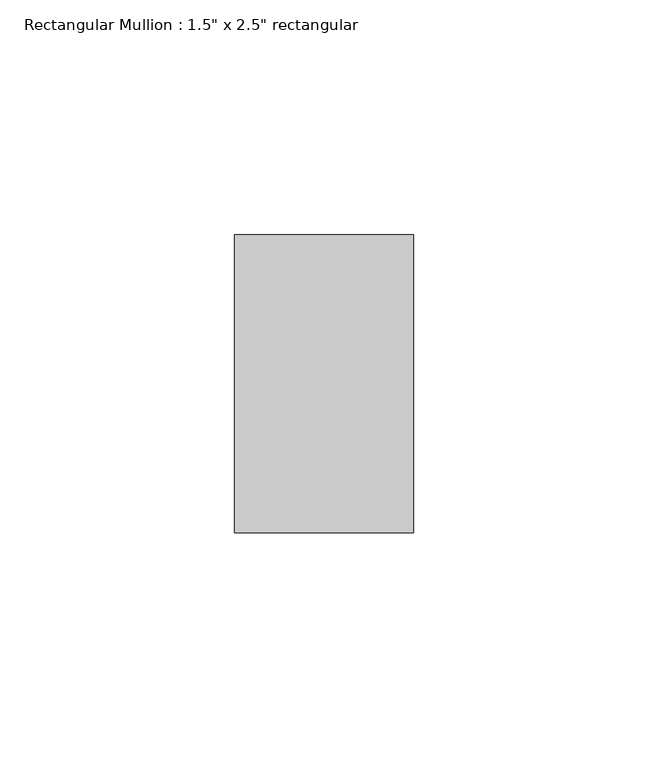
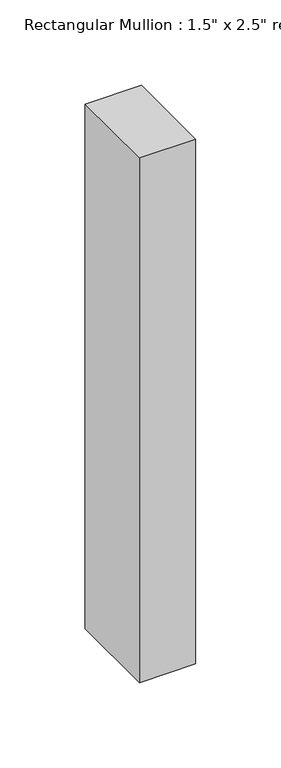
"""IFC4 building model written with IfcOpenShell, lengths in millimetres: member geometry."""

from ifc_helpers import new_model, si_unit, frame, origin, place, context, project, spatial, polyline, outline, extrude, source, transform, mapped, element, save


def member_89338317(model_context):
    return source(origin(), model_context, "Body", "SweptSolid", [
        extrude(outline(polyline([(0.0, 31.75), (0.0, -31.75), (-38.1, -31.75), (-38.1, 31.75), (0.0, 31.75)])), frame((0.0, 0.0, -375.1532928), z_axis=(0.0, 0.0, 1.0), x_axis=(1.0, 0.0, 0.0)), (0.0, 0.0, 1.0), 375.1532928),
    ])


if __name__ == "__main__":
    model = new_model("IFC4")
    model_context = context("Model", 3, world=origin())
    ifc_project = project(units=[si_unit("LENGTHUNIT", "METRE", prefix="MILLI")], contexts=[model_context])
    site = spatial("IfcSite", under=ifc_project)
    building = spatial("IfcBuilding", under=site)
    placement = place(None, origin())
    member_shape = member_89338317(model_context)
    element("IfcMember", 1, ObjectType="Rectangular Mullion : 1.5\" x 2.5\" rectangular", at=placement, inside=building, context=model_context, shape_type="MappedRepresentation", body=[
        mapped(member_shape, transform((0.0, 0.0, 0.0), x_axis=(1.0, 0.0, 0.0), y_axis=(0.0, 1.0, 0.0), z_axis=(0.0, 0.0, 1.0))),
    ])
    save(model, "model.ifc")

# Revit data of these elements
# Type "Rectangular Mullion : 1.5\" x 2.5\" rectangular"
#   built-in parameter 1007304 = 0.208333 (stored number, unit not read)
#   built-in parameter 1007301 = 0.0625 (stored number, unit not read)
#   built-in parameter 1007300 = 0.0625 (stored number, unit not read)
# Element 1 (IfcMember, "Rectangular Mullion : 1.5\" x 2.5\" rectangular")
#   Materials on its faces: "Aluminum"
# Materials
#   "Aluminum": class "Metal", colour RGB 247 247 247, transparency 0, Description = "Aluminum 6061", Cost = 0
